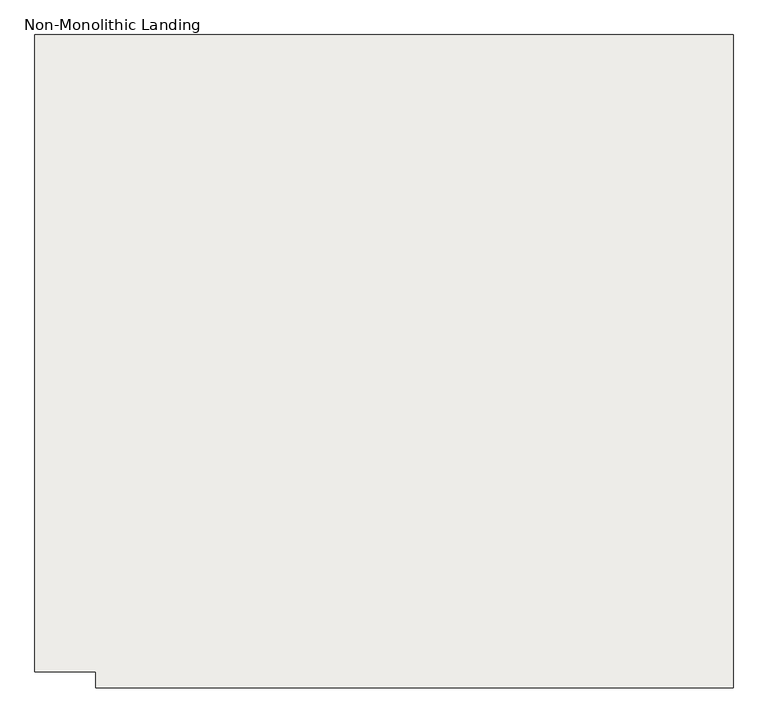
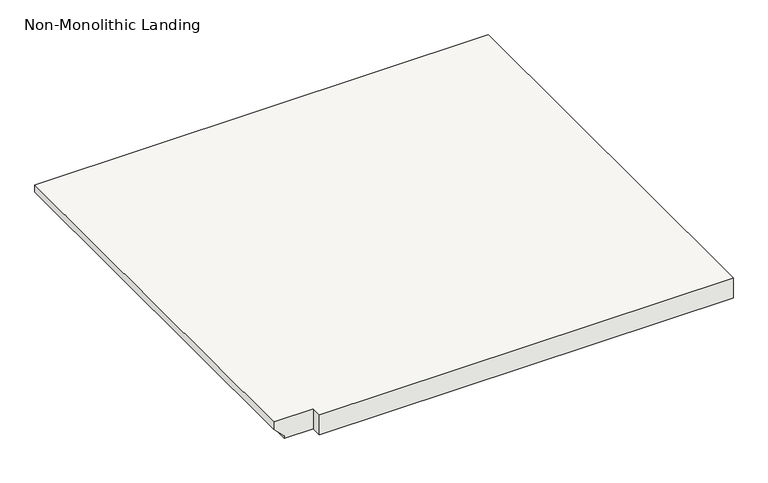
"""IFC4 building model written with IfcOpenShell, lengths in millimetres: slab geometry, Non-Monolithic Landing."""

from ifc_helpers import new_model, si_unit, origin, place, context, project, spatial, faceted_brep, source, transform, mapped, element, save


def non_monolithic_landing_135483eb(model_context):
    return source(origin(), model_context, "Body", "Brep", [
        faceted_brep([(-5053.3502524, 11195.5128362, 2266.95), (-5053.3502524, 11195.5128362, 2286.0), (-5053.3502524, 12192.4628362, 2286.0), (-5053.3502524, 12192.4628362, 2266.95), (-5027.9502524, 11195.5128362, 2241.55), (-5027.9502524, 12192.4628362, 2241.55), (-4958.1002526, 11195.5128362, 2286.0), (-4958.1002526, 11170.1128362, 2286.0), (-3961.1502526, 11170.1128362, 2286.0), (-3961.1502526, 11195.5128362, 2286.0), (-3961.1502526, 12192.4628362, 2286.0), (-5027.9502524, 11195.5128362, 2235.2), (-5027.9502524, 12192.4628362, 2235.2), (-3961.1502526, 12192.4628362, 2235.2), (-3961.1502526, 11195.5128362, 2235.2), (-3961.1502526, 11170.1128362, 2235.2), (-4958.1002526, 11170.1128362, 2235.2), (-4958.1002526, 11195.5128362, 2235.2)], [[[0, 1, 2, 3]], [[4, 0, 3, 5]], [[6, 7, 8, 9, 10, 2, 1]], [[11, 12, 13, 14, 15, 16, 17]], [[12, 11, 4, 5]], [[6, 1, 0, 4, 11, 17]], [[7, 6, 17, 16]], [[8, 7, 16, 15]], [[9, 8, 15, 14]], [[10, 9, 14, 13]], [[2, 10, 13, 12, 5, 3]]]),
    ])


if __name__ == "__main__":
    model = new_model("IFC4")
    model_context = context("Model", 3, world=origin())
    ifc_project = project(units=[si_unit("LENGTHUNIT", "METRE", prefix="MILLI")], contexts=[model_context])
    site = spatial("IfcSite", under=ifc_project)
    building = spatial("IfcBuilding", under=site)
    placement = place(None, origin())
    non_monolithic_landing_shape = non_monolithic_landing_135483eb(model_context)
    element("IfcSlab", 1, ObjectType="Non-Monolithic Landing", at=placement, inside=building, context=model_context, shape_type="MappedRepresentation", body=[
        mapped(non_monolithic_landing_shape, transform((0.0, 0.0, 0.0), x_axis=(1.0, 0.0, 0.0), y_axis=(0.0, 1.0, 0.0), z_axis=(0.0, 0.0, 1.0))),
    ])
    save(model, "model.ifc")
